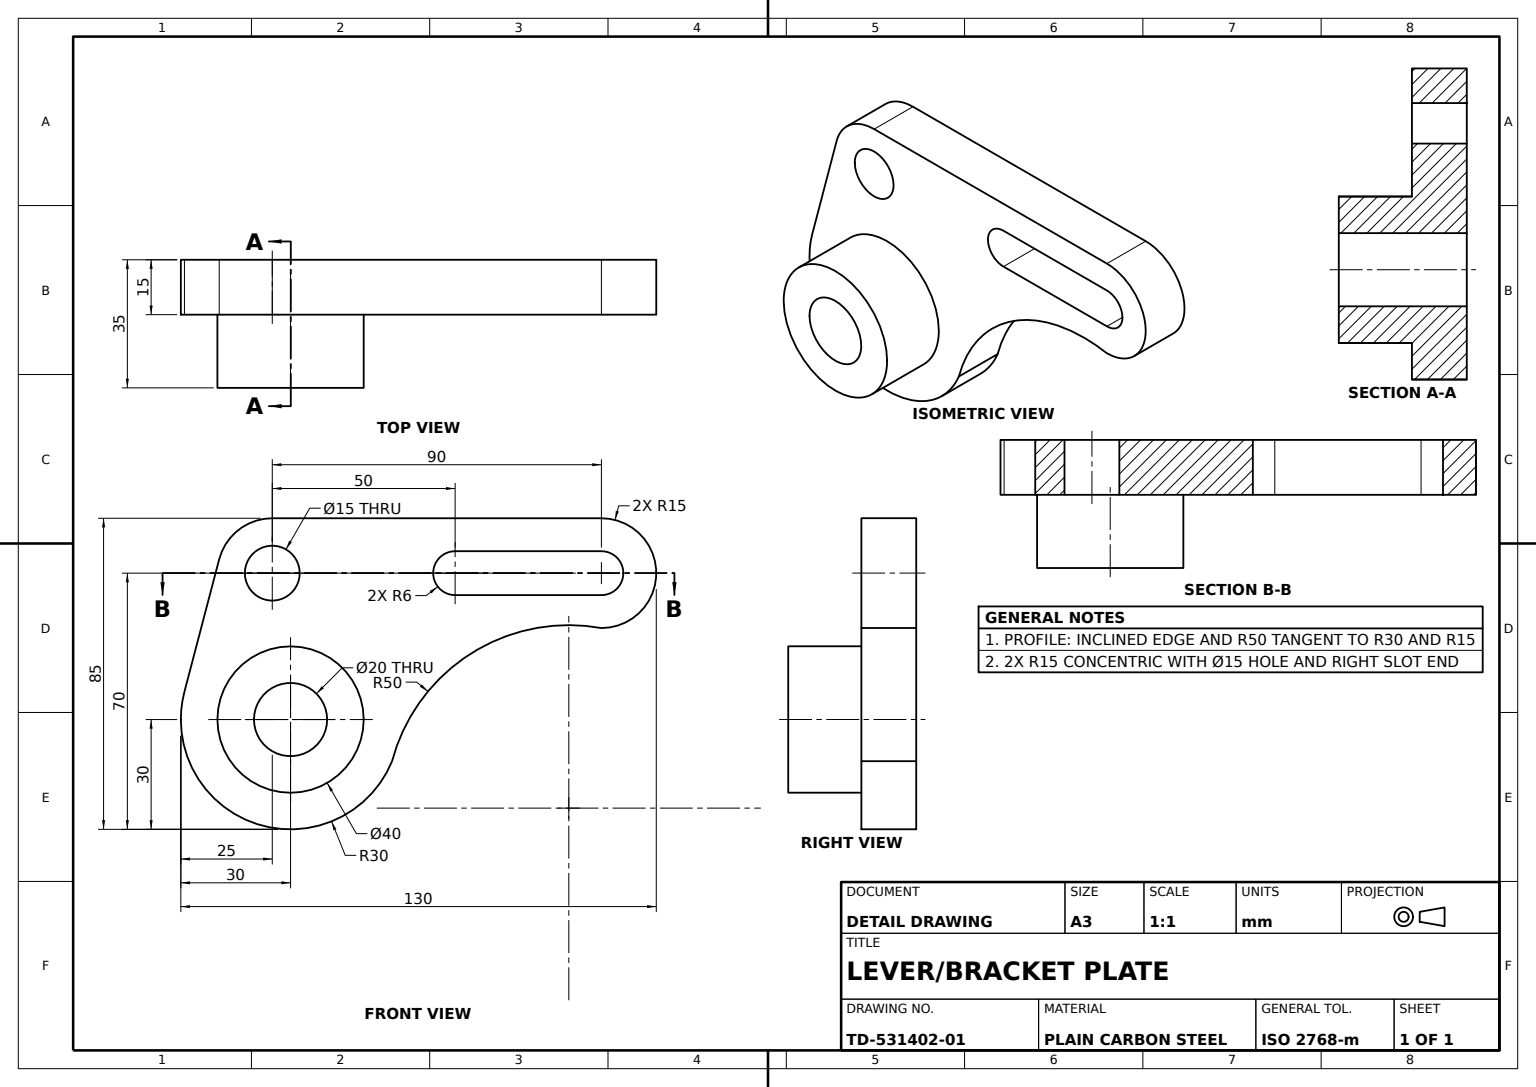
from build123d import *

# Parameters (mm, degrees)
LEVER_PLATE_DEPTH  = 15
HUB_PROFILE_R      = 20
HUB_40_DEPTH       = 20
HUB_BORE_PROFILE_R = 10
HUB_BORE_20_DEPTH  = 35
HOLE_PROFILE_R     = 7.5
HOLE_15_DEPTH      = 15
SLOT_12MM_DEPTH    = 15


with BuildPart() as part:
    # Lever Plate Profile → Lever Plate (new body)
    with BuildSketch(Plane.XY):
        with BuildLine():
            Line((15, 0), (105, 0))
            ThreePointArc((105, 0), (120, -15), (105, -30))
            ThreePointArc((105, -30), (69.260667374, -37.003214388), (47.752561519, -66.392775304))
            ThreePointArc((47.752561519, -66.392775304), (10.471129254, -83.44645184), (-9.015316087, -47.376914511))
            Line((-9.015316087, -47.376914511), (0.492341957, -11.188457255))
            ThreePointArc((0.492341957, -11.188457255), (5.83957264, -3.122013193), (15, 0))
        make_face()
    extrude(amount=LEVER_PLATE_DEPTH)

    # Hub Profile → Hub Ø40 (add)
    with BuildSketch(Plane.XY.offset(15)):
        with Locations((20, -55)):
            Circle(HUB_PROFILE_R)
    extrude(amount=HUB_40_DEPTH)

    # Hub Bore Profile → Hub Bore Ø20 (cut)
    with BuildSketch(Plane.XY.offset(35)):
        with Locations((20, -55)):
            Circle(HUB_BORE_PROFILE_R)
    extrude(amount=-HUB_BORE_20_DEPTH, mode=Mode.SUBTRACT)

    # Hole Profile → Hole Ø15 (cut)
    with BuildSketch(Plane.XY.offset(15)):
        with Locations((15, -15)):
            Circle(HOLE_PROFILE_R)
    extrude(amount=-HOLE_15_DEPTH, mode=Mode.SUBTRACT)

    # Slot Profile → Slot 12mm (cut)
    with BuildSketch(Plane.XY.offset(15)):
        with BuildLine():
            Line((65, -9), (105, -9))
            ThreePointArc((105, -9), (111, -15), (105, -21))
            Line((105, -21), (65, -21))
            ThreePointArc((65, -21), (59, -15), (65, -9))
        make_face()
    extrude(amount=-SLOT_12MM_DEPTH, mode=Mode.SUBTRACT)


solid = part.part
